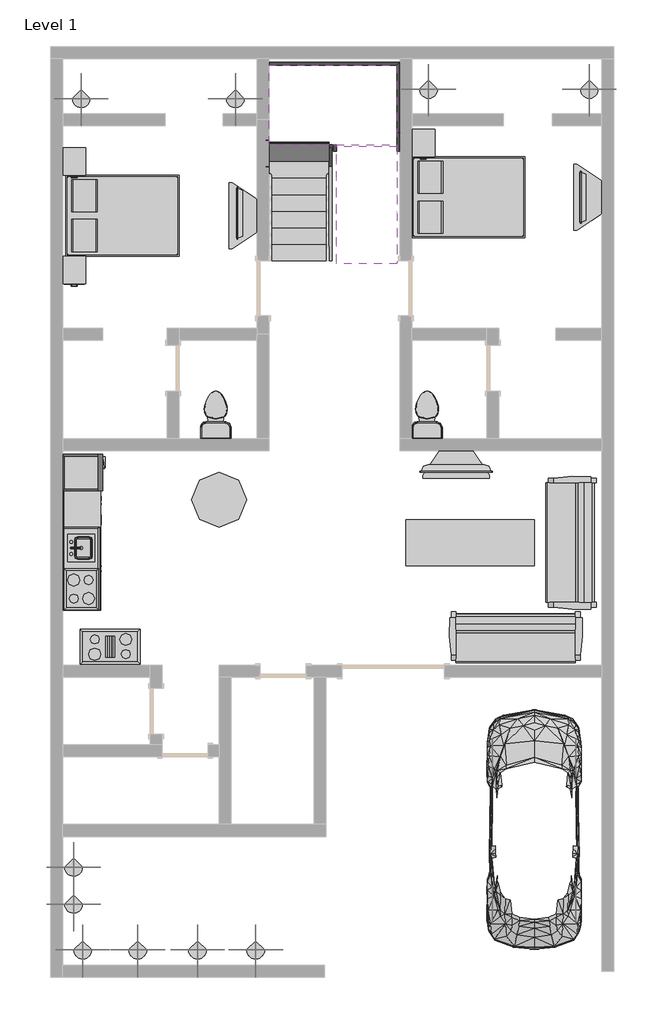
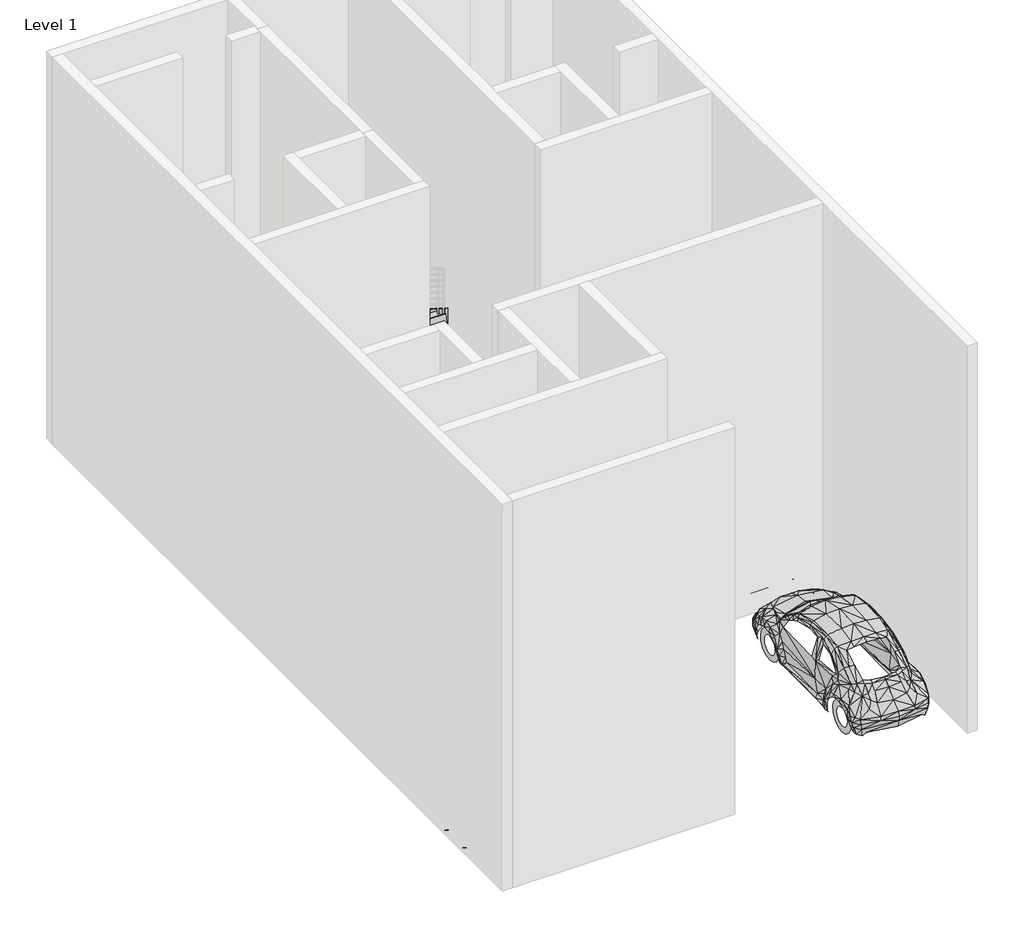
# One storey, part 4 of 4: 16 furniture elements, 10 geographic elements, 8 members, 6 proxies, 3 flow terminals, 2 stair flights, 1 slab.
"""IFC4 building model written with IfcOpenShell, lengths in millimetres."""

from ifc_helpers import new_model, si_unit, frame, origin, place, context, project, spatial, polyline, outline, extrude, faceted_brep, transform, mapped, element, save
from components import m_cook_top_4_unit_0915_x_500mm_0d6b06ed, m_cook_top_4_unit2_0615_x_500mm_249f3515, m_dishwasher_610_x_610_x_875mm_54ecfc4c, m_kitchenette_medium_1372mm_e05c6bec, m_rpc_beetle_m_rpc_beetle_b6d71803, m_refrigerator_600_x_660mm_a466bf94, m_sink_kitchen_island_450_x_450mm_f969cf2d, m_toilet_domestic_3d_m_toilet_domestic_3d_5cb52bd4, m_toilet_domestic_3d_m_toilet_domestic_3d_183bbd19, furniture_40ec15d9, furniture_0810mm_56245f3a, furniture_1190mm_d9bcc661, m_bed_box_1346_x_1880mm_double_b32eb57e, m_cabinet_file_2_drawer_0380_x_0457mm_9eec7cff, m_counter_top_w_sink_hole_600mm_depth_0a237b63, m_sofa_pensi_2134mm_91f3548c, m_table_dining_0762_x_2134mm_3327233b, m_table_dining_round_w_chairs_0915mm_diameter_5defa876, m_rpc_plant_tropical_agave_0_45_meters_eb57889b, non_monolithic_landing_64e54c11, stair_flight_50mm_tread_25mm_nosing_13mm_riser_88d6afc4, stair_flight_50mm_tread_25mm_nosing_13mm_riser_daaaf0ad

model = new_model("IFC4")

# Units and contexts
model_context = context("Model", 3, world=origin())
ifc_project = project(units=[si_unit("LENGTHUNIT", "METRE", prefix="MILLI")], contexts=[model_context])

# Site, building, storey
site = spatial("IfcSite", under=ifc_project)
building = spatial("IfcBuilding", under=site)
storey = spatial("IfcBuildingStorey", under=building, Name="Level 1", Elevation=0.0)

# Proxies
placement = place(None, origin())
m_cook_top_4_unit_0915_x_500mm_shape = m_cook_top_4_unit_0915_x_500mm_0d6b06ed(model_context)
element("IfcBuildingElementProxy", 1, Name="M_Cook Top-4 Unit : 0915 x 500mm", ObjectType="M_Cook Top-4 Unit : 0915 x 500mm", at=placement, inside=storey, context=model_context, shape_type="MappedRepresentation", body=[
    mapped(m_cook_top_4_unit_0915_x_500mm_shape, transform((-7196.5697318, 2497.9482221, 0.0), x_axis=(1.0, 0.0, 0.0), y_axis=(0.0, 1.0, 0.0), z_axis=(0.0, 0.0, 1.0))),
])
m_cook_top_4_unit2_0615_x_500mm_shape = m_cook_top_4_unit2_0615_x_500mm_249f3515(model_context)
element("IfcBuildingElementProxy", 2, Name="M_Cook Top-4 Unit2 : 0615 x 500mm", ObjectType="M_Cook Top-4 Unit2 : 0615 x 500mm", at=placement, inside=storey, context=model_context, shape_type="MappedRepresentation", body=[
    mapped(m_cook_top_4_unit2_0615_x_500mm_shape, transform((-7678.9697318, 3450.1482221, 0.0), x_axis=(0.0, 1.0000000000000002, 0.0), y_axis=(-1.0000000000000002, 0.0, 0.0), z_axis=(0.0, 0.0, 1.0))),
])
m_dishwasher_610_x_610_x_875mm_shape = m_dishwasher_610_x_610_x_875mm_54ecfc4c(model_context)
element("IfcBuildingElementProxy", 3, Name="M_Dishwasher : 610 x 610 x 875mm", ObjectType="M_Dishwasher : 610 x 610 x 875mm", at=placement, inside=storey, context=model_context, shape_type="MappedRepresentation", body=[
    mapped(m_dishwasher_610_x_610_x_875mm_shape, transform((-7412.320167, 4399.6307536, 0.0), x_axis=(0.0, 1.0000000000000002, 0.0), y_axis=(-1.0000000000000002, 0.0, 0.0), z_axis=(0.0, 0.0, 1.0))),
])
m_kitchenette_medium_1372mm_shape = m_kitchenette_medium_1372mm_e05c6bec(model_context)
element("IfcBuildingElementProxy", 4, Name="M_Kitchenette - Medium : 1372mm", ObjectType="M_Kitchenette - Medium : 1372mm", at=placement, inside=storey, context=model_context, shape_type="MappedRepresentation", body=[
    mapped(m_kitchenette_medium_1372mm_shape, transform((-7983.9697318, 3774.4105172, 0.0), x_axis=(0.0, 1.0000000000000002, 0.0), y_axis=(-1.0000000000000002, 0.0, 0.0), z_axis=(0.0, 0.0, 1.0))),
])
m_rpc_beetle_m_rpc_beetle_shape = m_rpc_beetle_m_rpc_beetle_b6d71803(model_context)
element("IfcBuildingElementProxy", 5, Name="M_RPC Beetle : M_RPC Beetle", ObjectType="M_RPC Beetle : M_RPC Beetle", at=placement, inside=storey, context=model_context, shape_type="MappedRepresentation", body=[
    mapped(m_rpc_beetle_m_rpc_beetle_shape, transform((-159.1697318, -1769.2517779, 0.0), x_axis=(1.0, 0.0, 0.0), y_axis=(0.0, 1.0, 0.0), z_axis=(0.0, 0.0, 1.0))),
])
m_refrigerator_600_x_660mm_shape = m_refrigerator_600_x_660mm_a466bf94(model_context)
element("IfcBuildingElementProxy", 6, Name="M_Refrigerator : 600 x 660mm", ObjectType="M_Refrigerator : 600 x 660mm", at=placement, inside=storey, context=model_context, shape_type="MappedRepresentation", body=[
    mapped(m_refrigerator_600_x_660mm_shape, transform((-7687.7546416, 5440.9493647, 0.0), x_axis=(0.0, 1.0000000000000002, 0.0), y_axis=(-1.0000000000000002, 0.0, 0.0), z_axis=(0.0, 0.0, 1.0))),
])

# Flow terminals
m_sink_kitchen_island_450_x_450mm_shape = m_sink_kitchen_island_450_x_450mm_f969cf2d(model_context)
element("IfcFlowTerminal", 7, ObjectType="M_Sink Kitchen-Island : 450 x 450mm", at=placement, inside=storey, context=model_context, shape_type="MappedRepresentation", body=[
    mapped(m_sink_kitchen_island_450_x_450mm_shape, transform((-7676.6243307, 4120.4589815, 0.0), x_axis=(0.0, 1.0000000000000002, 0.0), y_axis=(-1.0000000000000002, 0.0, 0.0), z_axis=(0.0, 0.0, 1.0))),
])
m_toilet_domestic_3d_m_toilet_domestic_3d_shape = m_toilet_domestic_3d_m_toilet_domestic_3d_5cb52bd4(model_context)
m_toilet_domestic_3d_m_toilet_domestic_3d_2_shape = m_toilet_domestic_3d_m_toilet_domestic_3d_183bbd19(model_context)
element("IfcFlowTerminal", 8, ObjectType="M_Toilet-Domestic-3D : M_Toilet-Domestic-3D", at=placement, inside=storey, context=model_context, shape_type="MappedRepresentation", body=[
    mapped(m_toilet_domestic_3d_m_toilet_domestic_3d_shape, transform((-1937.7737045, 6434.9482221, 0.0), x_axis=(-1.0, 0.0, 0.0), y_axis=(0.0, -1.0, 0.0), z_axis=(0.0, 0.0, 1.0))),
    mapped(m_toilet_domestic_3d_m_toilet_domestic_3d_2_shape, transform((-1937.7737045, 6434.9482221, 0.0), x_axis=(-1.0, 0.0, 0.0), y_axis=(0.0, -1.0, 0.0), z_axis=(0.0, 0.0, 1.0))),
])
element("IfcFlowTerminal", 9, ObjectType="M_Toilet-Domestic-3D : M_Toilet-Domestic-3D", at=placement, inside=storey, context=model_context, shape_type="MappedRepresentation", body=[
    mapped(m_toilet_domestic_3d_m_toilet_domestic_3d_shape, transform((-5444.9657592, 6434.9482221, 0.0), x_axis=(-1.0, 0.0, 0.0), y_axis=(0.0, -1.0, 0.0), z_axis=(0.0, 0.0, 1.0))),
    mapped(m_toilet_domestic_3d_m_toilet_domestic_3d_2_shape, transform((-5444.9657592, 6434.9482221, 0.0), x_axis=(-1.0, 0.0, 0.0), y_axis=(0.0, -1.0, 0.0), z_axis=(0.0, 0.0, 1.0))),
])

# Furniture
furniture_shape = furniture_40ec15d9(model_context)
element("IfcFurniture", 10, at=placement, inside=storey, context=model_context, shape_type="MappedRepresentation", body=[
    mapped(furniture_shape, transform((-4761.3197318, 9773.3362242, 0.0), x_axis=(0.0, -1.0000000000000002, 0.0), y_axis=(1.0000000000000002, 0.0, 0.0), z_axis=(0.0, 0.0, 1.0))),
])
element("IfcFurniture", 11, at=placement, inside=storey, context=model_context, shape_type="MappedRepresentation", body=[
    mapped(furniture_shape, transform((960.0302682, 10078.1362242, 0.0), x_axis=(0.0, -1.0, 0.0), y_axis=(1.0, 0.0, 0.0), z_axis=(0.0, 0.0, 1.0))),
])
element("IfcFurniture", 12, at=placement, inside=storey, context=model_context, shape_type="MappedRepresentation", body=[
    mapped(furniture_shape, transform((-1579.7577339, 5750.7482221, 0.0), x_axis=(1.0, 0.0, 0.0), y_axis=(0.0, 1.0, 0.0), z_axis=(0.0, 0.0, 1.0))),
])
furniture_0810mm_shape = furniture_0810mm_56245f3a(model_context)
element("IfcFurniture", 13, ObjectType="0810mm", at=placement, inside=storey, context=model_context, shape_type="MappedRepresentation", body=[
    mapped(furniture_0810mm_shape, transform((671.4916445, 9949.0037079, 0.0), x_axis=(0.0, -1.0000000000000004, 0.0), y_axis=(1.0000000000000004, 0.0, 0.0), z_axis=(0.0, 0.0, 1.0))),
])
element("IfcFurniture", 14, ObjectType="0810mm", at=placement, inside=storey, context=model_context, shape_type="MappedRepresentation", body=[
    mapped(furniture_0810mm_shape, transform((-5028.259817, 9682.2037079, 0.0), x_axis=(0.0, -1.0, 0.0), y_axis=(1.0, 0.0, 0.0), z_axis=(0.0, 0.0, 1.0))),
])
furniture_1190mm_shape = furniture_1190mm_d9bcc661(model_context)
element("IfcFurniture", 15, ObjectType="1190mm", at=placement, inside=storey, context=model_context, shape_type="MappedRepresentation", body=[
    mapped(furniture_1190mm_shape, transform((-1450.6252177, 5462.2095984, 0.0), x_axis=(1.0, 0.0, 0.0), y_axis=(0.0, 1.0, 0.0), z_axis=(0.0, 0.0, 1.0))),
])
m_bed_box_1346_x_1880mm_double_shape = m_bed_box_1346_x_1880mm_double_b32eb57e(model_context)
element("IfcFurniture", 16, ObjectType="M_Bed-Box : 1346 x 1880mm - Double", at=placement, inside=storey, context=model_context, shape_type="MappedRepresentation", body=[
    mapped(m_bed_box_1346_x_1880mm_double_shape, transform((-7229.59924, 9308.9957631, 0.0), x_axis=(0.0, 1.0, 0.0), y_axis=(-1.0, 0.0, 0.0), z_axis=(0.0, 0.0, 1.0))),
])
element("IfcFurniture", 17, ObjectType="M_Bed-Box : 1346 x 1880mm - Double", at=placement, inside=storey, context=model_context, shape_type="MappedRepresentation", body=[
    mapped(m_bed_box_1346_x_1880mm_double_shape, transform((-1485.59924, 9613.7957631, 0.0), x_axis=(0.0, 1.0, 0.0), y_axis=(-1.0, 0.0, 0.0), z_axis=(0.0, 0.0, 1.0))),
])
m_cabinet_file_2_drawer_0380_x_0457mm_shape = m_cabinet_file_2_drawer_0380_x_0457mm_9eec7cff(model_context)
element("IfcFurniture", 18, ObjectType="M_Cabinet-File 2 Drawer : 0380 x 0457mm", at=placement, inside=storey, context=model_context, shape_type="MappedRepresentation", body=[
    mapped(m_cabinet_file_2_drawer_0380_x_0457mm_shape, transform((-7666.0732848, 10691.7825222, 0.0), x_axis=(1.0, 0.0, 0.0), y_axis=(0.0, 1.0, 0.0), z_axis=(0.0, 0.0, 1.0))),
])
element("IfcFurniture", 19, ObjectType="M_Cabinet-File 2 Drawer : 0380 x 0457mm", at=placement, inside=storey, context=model_context, shape_type="MappedRepresentation", body=[
    mapped(m_cabinet_file_2_drawer_0380_x_0457mm_shape, transform((-7666.0732848, 8888.7825222, 0.0), x_axis=(1.0, 0.0, 0.0), y_axis=(0.0, 1.0, 0.0), z_axis=(0.0, 0.0, 1.0))),
])
element("IfcFurniture", 20, ObjectType="M_Cabinet-File 2 Drawer : 0380 x 0457mm", at=placement, inside=storey, context=model_context, shape_type="MappedRepresentation", body=[
    mapped(m_cabinet_file_2_drawer_0380_x_0457mm_shape, transform((-1873.2732848, 10996.5825222, 0.0), x_axis=(1.0, 0.0, 0.0), y_axis=(0.0, 1.0, 0.0), z_axis=(0.0, 0.0, 1.0))),
])
m_counter_top_w_sink_hole_600mm_depth_shape = m_counter_top_w_sink_hole_600mm_depth_0a237b63(model_context)
element("IfcFurniture", 21, ObjectType="M_Counter Top w Sink Hole : 600mm Depth", at=placement, inside=storey, context=model_context, shape_type="MappedRepresentation", body=[
    mapped(m_counter_top_w_sink_hole_600mm_depth_shape, transform((-7983.9697318, 4307.6105172, 0.0), x_axis=(0.0, 1.0000000000000002, 0.0), y_axis=(-1.0000000000000002, 0.0, 0.0), z_axis=(0.0, 0.0, 1.0))),
])
m_sofa_pensi_2134mm_shape = m_sofa_pensi_2134mm_91f3548c(model_context)
element("IfcFurniture", 22, ObjectType="M_Sofa-Pensi : 2134mm", at=placement, inside=storey, context=model_context, shape_type="MappedRepresentation", body=[
    mapped(m_sofa_pensi_2134mm_shape, transform((173.3204321, 4502.1544721, 0.0), x_axis=(0.0, -1.0000000000000004, 0.0), y_axis=(1.0000000000000004, 0.0, 0.0), z_axis=(0.0, 0.0, 1.0))),
])
element("IfcFurniture", 23, ObjectType="M_Sofa-Pensi : 2134mm", at=placement, inside=storey, context=model_context, shape_type="MappedRepresentation", body=[
    mapped(m_sofa_pensi_2134mm_shape, transform((-742.5759818, 2373.238386, 0.0), x_axis=(1.0, 0.0, 0.0), y_axis=(0.0, 1.0, 0.0), z_axis=(0.0, 0.0, 1.0))),
])
m_table_dining_0762_x_2134mm_shape = m_table_dining_0762_x_2134mm_3327233b(model_context)
element("IfcFurniture", 24, ObjectType="M_Table-Dining : 0762 x 2134mm", at=placement, inside=storey, context=model_context, shape_type="MappedRepresentation", body=[
    mapped(m_table_dining_0762_x_2134mm_shape, transform((-1206.1039651, 4318.7592999, 0.0), x_axis=(-1.0, 0.0, 0.0), y_axis=(0.0, -1.0, 0.0), z_axis=(0.0, 0.0, 1.0))),
])
m_table_dining_round_w_chairs_0915mm_diameter_shape = m_table_dining_round_w_chairs_0915mm_diameter_5defa876(model_context)
element("IfcFurniture", 25, ObjectType="M_Table-Dining Round w Chairs : 0915mm Diameter", at=placement, inside=storey, context=model_context, shape_type="MappedRepresentation", body=[
    mapped(m_table_dining_round_w_chairs_0915mm_diameter_shape, transform((-5495.251699, 5121.2269106, 0.0), x_axis=(1.0, 0.0, 0.0), y_axis=(0.0, 1.0, 0.0), z_axis=(0.0, 0.0, 1.0))),
])

# Geographic elements
m_rpc_plant_tropical_agave_0_45_meters_shape = m_rpc_plant_tropical_agave_0_45_meters_eb57889b(model_context)
element("IfcGeographicElement", 26, ObjectType="M_RPC Plant - Tropical : Agave - 0.45 Meters", at=placement, inside=storey, context=model_context, shape_type="MappedRepresentation", body=[
    mapped(m_rpc_plant_tropical_agave_0_45_meters_shape, transform((-7653.9664029, -2531.2517779, 0.0), x_axis=(1.0, 0.0, 0.0), y_axis=(0.0, 1.0, 0.0), z_axis=(0.0, 0.0, 1.0))),
])
element("IfcGeographicElement", 27, ObjectType="M_RPC Plant - Tropical : Agave - 0.45 Meters", at=placement, inside=storey, context=model_context, shape_type="MappedRepresentation", body=[
    mapped(m_rpc_plant_tropical_agave_0_45_meters_shape, transform((-6739.5664029, -2531.2517779, 0.0), x_axis=(1.0, 0.0, 0.0), y_axis=(0.0, 1.0, 0.0), z_axis=(0.0, 0.0, 1.0))),
])
element("IfcGeographicElement", 28, ObjectType="M_RPC Plant - Tropical : Agave - 0.45 Meters", at=placement, inside=storey, context=model_context, shape_type="MappedRepresentation", body=[
    mapped(m_rpc_plant_tropical_agave_0_45_meters_shape, transform((-5748.9664029, -2531.2517779, 0.0), x_axis=(1.0, 0.0, 0.0), y_axis=(0.0, 1.0, 0.0), z_axis=(0.0, 0.0, 1.0))),
])
element("IfcGeographicElement", 29, ObjectType="M_RPC Plant - Tropical : Agave - 0.45 Meters", at=placement, inside=storey, context=model_context, shape_type="MappedRepresentation", body=[
    mapped(m_rpc_plant_tropical_agave_0_45_meters_shape, transform((-4782.1664029, -2531.2517779, 0.0), x_axis=(1.0, 0.0, 0.0), y_axis=(0.0, 1.0, 0.0), z_axis=(0.0, 0.0, 1.0))),
])
element("IfcGeographicElement", 30, ObjectType="M_RPC Plant - Tropical : Agave - 0.45 Meters", at=placement, inside=storey, context=model_context, shape_type="MappedRepresentation", body=[
    mapped(m_rpc_plant_tropical_agave_0_45_meters_shape, transform((-7806.3664029, -1159.6517779, 0.0), x_axis=(1.0, 0.0, 0.0), y_axis=(0.0, 1.0, 0.0), z_axis=(0.0, 0.0, 1.0))),
])
element("IfcGeographicElement", 31, ObjectType="M_RPC Plant - Tropical : Agave - 0.45 Meters", at=placement, inside=storey, context=model_context, shape_type="MappedRepresentation", body=[
    mapped(m_rpc_plant_tropical_agave_0_45_meters_shape, transform((-7806.3664029, -1769.2517779, 0.0), x_axis=(1.0, 0.0, 0.0), y_axis=(0.0, 1.0, 0.0), z_axis=(0.0, 0.0, 1.0))),
])
element("IfcGeographicElement", 32, ObjectType="M_RPC Plant - Tropical : Agave - 0.45 Meters", at=placement, inside=storey, context=model_context, shape_type="MappedRepresentation", body=[
    mapped(m_rpc_plant_tropical_agave_0_45_meters_shape, transform((-7679.3664029, 11591.1482221, 0.0), x_axis=(1.0, 0.0, 0.0), y_axis=(0.0, 1.0, 0.0), z_axis=(0.0, 0.0, 1.0))),
])
element("IfcGeographicElement", 33, ObjectType="M_RPC Plant - Tropical : Agave - 0.45 Meters", at=placement, inside=storey, context=model_context, shape_type="MappedRepresentation", body=[
    mapped(m_rpc_plant_tropical_agave_0_45_meters_shape, transform((-5120.3164029, 11591.1482221, 0.0), x_axis=(1.0, 0.0, 0.0), y_axis=(0.0, 1.0, 0.0), z_axis=(0.0, 0.0, 1.0))),
])
element("IfcGeographicElement", 34, ObjectType="M_RPC Plant - Tropical : Agave - 0.45 Meters", at=placement, inside=storey, context=model_context, shape_type="MappedRepresentation", body=[
    mapped(m_rpc_plant_tropical_agave_0_45_meters_shape, transform((-1911.9664029, 11743.5482221, 0.0), x_axis=(1.0, 0.0, 0.0), y_axis=(0.0, 1.0, 0.0), z_axis=(0.0, 0.0, 1.0))),
])
element("IfcGeographicElement", 35, ObjectType="M_RPC Plant - Tropical : Agave - 0.45 Meters", at=placement, inside=storey, context=model_context, shape_type="MappedRepresentation", body=[
    mapped(m_rpc_plant_tropical_agave_0_45_meters_shape, transform((755.0335971, 11743.5482221, 0.0), x_axis=(1.0, 0.0, 0.0), y_axis=(0.0, 1.0, 0.0), z_axis=(0.0, 0.0, 1.0))),
])

# Members
element("IfcMember", 36, ObjectType="Stringer - 50mm Width", at=placement, inside=storey, context=model_context, shape_type="SweptSolid", body=[
    extrude(outline(polyline([(8898.7482221, 0.0), (8898.7482221, 215.089535), (10833.5792256, 1438.6980748), (10949.4482857, 1038.6980748), (9307.0069549, 0.0), (8898.7482221, 0.0)])), frame((-4612.9197318, 0.0, 0.0), z_axis=(1.0, 0.0, 0.0), x_axis=(0.0, 1.0, 0.0)), (0.0, 0.0, 1.0), 50.0),
])
element("IfcMember", 37, ObjectType="Stringer - 50mm Width", at=placement, inside=storey, context=model_context, shape_type="SweptSolid", body=[
    extrude(outline(polyline([(8898.7482221, 0.0), (8898.7482221, 215.089535), (10773.7482221, 1400.860286), (10773.7482221, 927.5834101), (9307.0069549, 0.0), (8898.7482221, 0.0)])), frame((-3562.8939506, 0.0, 0.0), z_axis=(1.0, 0.0, 0.0), x_axis=(0.0, 1.0, 0.0)), (0.0, 0.0, 1.0), 50.0),
])
element("IfcMember", 38, ObjectType="Stringer - 50mm Width", at=placement, inside=storey, context=model_context, shape_type="SweptSolid", body=[
    extrude(outline(polyline([(11088.9172185, 1438.6980748), (10973.0481585, 1038.6980748), (8898.7482221, 2350.5083113), (8898.7482221, 2823.7851872), (11088.9172185, 1438.6980748)])), frame((-2440.2681693, 0.0, 0.0), z_axis=(1.0, 0.0, 0.0), x_axis=(0.0, 1.0, 0.0)), (0.0, 0.0, 1.0), 50.0),
])
element("IfcMember", 39, ObjectType="Stringer - 50mm Width", at=placement, inside=storey, context=model_context, shape_type="SweptSolid", body=[
    extrude(outline(polyline([(10823.7482221, 1606.3938828), (10823.7482221, 1133.1170069), (8898.7482221, 2350.5083113), (8898.7482221, 2823.7851872), (10823.7482221, 1606.3938828)])), frame((-3490.2939506, 0.0, 0.0), z_axis=(1.0, 0.0, 0.0), x_axis=(0.0, 1.0, 0.0)), (0.0, 0.0, 1.0), 50.0),
])
element("IfcMember", 40, ObjectType="Stringer - 50mm Width", at=placement, inside=storey, context=model_context, shape_type="Brep", body=[
    faceted_brep([(-2440.2681693, 11088.9172185, 1438.6980748), (-2390.2681693, 11088.9172185, 1438.6980748), (-2390.2681693, 12194.5482221, 1438.6980748), (-2440.2681693, 12144.5482221, 1438.6980748), (-2440.2681693, 10973.0481585, 1038.6980748), (-2440.2681693, 12144.5482221, 1038.6980748), (-2390.2681693, 10973.0481585, 1038.6980748), (-2390.2681693, 12194.5482221, 1038.6980748)], [[[0, 1, 2, 3]], [[4, 0, 3, 5]], [[6, 4, 5, 7]], [[1, 6, 7, 2]], [[1, 0, 4, 6]], [[2, 7, 5, 3]]]),
])
element("IfcMember", 41, ObjectType="Stringer - 50mm Width", at=placement, inside=storey, context=model_context, shape_type="SweptSolid", body=[
    extrude(outline(polyline([(-2390.2681693, 12194.5482221), (-2440.2681693, 12144.5482221), (-4562.9197318, 12144.5482221), (-4612.9197318, 12194.5482221), (-2390.2681693, 12194.5482221)])), frame((0.0, 0.0, 1038.6980748), z_axis=(0.0, 0.0, 1.0), x_axis=(1.0, 0.0, 0.0)), (0.0, 0.0, 1.0), 400.0),
])
element("IfcMember", 42, ObjectType="Stringer - 50mm Width", at=placement, inside=storey, context=model_context, shape_type="Brep", body=[
    faceted_brep([(-4562.9197318, 12144.5482221, 1438.6980748), (-4612.9197318, 12194.5482221, 1438.6980748), (-4612.9197318, 10833.5792256, 1438.6980748), (-4562.9197318, 10833.5792256, 1438.6980748), (-4562.9197318, 12144.5482221, 1038.6980748), (-4562.9197318, 10949.4482857, 1038.6980748), (-4612.9197318, 12194.5482221, 1038.6980748), (-4612.9197318, 10949.4482857, 1038.6980748)], [[[0, 1, 2, 3]], [[4, 0, 3, 5]], [[6, 4, 5, 7]], [[1, 6, 7, 2]], [[1, 0, 4, 6]], [[2, 7, 5, 3]]]),
])
element("IfcMember", 43, ObjectType="Stringer - 50mm Width", at=placement, inside=storey, context=model_context, shape_type="SweptSolid", body=[
    extrude(outline(polyline([(-3562.8939506, 10773.7482221), (-3562.8939506, 10823.7482221), (-3490.2939506, 10823.7482221), (-3490.2939506, 10773.7482221), (-3562.8939506, 10773.7482221)])), frame((0.0, 0.0, 1038.6980748), z_axis=(0.0, 0.0, 1.0), x_axis=(1.0, 0.0, 0.0)), (0.0, 0.0, 1.0), 400.0),
])

# Slab
non_monolithic_landing_shape = non_monolithic_landing_64e54c11(model_context)
element("IfcSlab", 44, ObjectType="Non-Monolithic Landing", at=placement, inside=storey, context=model_context, shape_type="MappedRepresentation", body=[
    mapped(non_monolithic_landing_shape, transform((0.0, 0.0, 0.0), x_axis=(1.0, 0.0, 0.0), y_axis=(0.0, 1.0, 0.0), z_axis=(0.0, 0.0, 1.0))),
])

# Stair flights
stair_flight_50mm_tread_25mm_nosing_13mm_riser_shape = stair_flight_50mm_tread_25mm_nosing_13mm_riser_88d6afc4(model_context)
element("IfcStairFlight", 45, ObjectType="50mm Tread 25mm Nosing 13mm Riser", at=placement, inside=storey, context=model_context, shape_type="MappedRepresentation", body=[
    mapped(stair_flight_50mm_tread_25mm_nosing_13mm_riser_shape, transform((0.0, 0.0, 0.0), x_axis=(1.0, 0.0, 0.0), y_axis=(0.0, 1.0, 0.0), z_axis=(0.0, 0.0, 1.0))),
])
stair_flight_50mm_tread_25mm_nosing_13mm_riser_2_shape = stair_flight_50mm_tread_25mm_nosing_13mm_riser_daaaf0ad(model_context)
element("IfcStairFlight", 46, ObjectType="50mm Tread 25mm Nosing 13mm Riser", at=placement, inside=storey, context=model_context, shape_type="MappedRepresentation", body=[
    mapped(stair_flight_50mm_tread_25mm_nosing_13mm_riser_2_shape, transform((0.0, 0.0, 0.0), x_axis=(1.0, 0.0, 0.0), y_axis=(0.0, 1.0, 0.0), z_axis=(0.0, 0.0, 1.0))),
])

save(model, "model.ifc")

# Revit data of these elements
# Type "M_Cook Top-4 Unit : 0915 x 500mm"
#   Counter Height = 900 mm
#   Depth = 500 mm
#   Width = 915 mm
#   Burner Material = Steel, Chrome Plated
#   Cooktop Material = Steel, Polished
#   Default Elevation = 0
# Type "M_Cook Top-4 Unit2 : 0615 x 500mm"
#   Depth = 500 mm
#   Width = 615 mm
#   Burner Material = Steel, Chrome Plated
#   Cooktop Material = Steel, Polished
#   Default Elevation = 0
#   Assembly Code = ""
# Type "M_Dishwasher : 610 x 610 x 875mm"
#   Label = "DW"
#   Depth = 610 mm
#   Height = 875 mm
#   Width = 610 mm
#   Dishwasher Material = Steel, Paint Finish, Ivory, Glossy
#   Panel Face Material = Plastic, Opaque Black
#   Default Elevation = 0
# Type "M_Kitchenette - Medium : 1372mm"
#   Counter Length = 1980 mm
#   Cabinet Width = 1372 mm
#   Cabinet Height = 900 mm
#   Cabinet Depth = 610 mm
#   Toe Depth = 35 mm
#   Toe Height = 100 mm
#   Cabinet Material = Cabinets
#   Door/Drawer Material = Cabinets
#   Handle Material = Cabinets - Handles
#   Default Elevation = 0
# Type "M_RPC Beetle : M_RPC Beetle"
#   built-in parameter 1005198 = "{2, 15},{39, RPC-16-0U6E-L4EG-ENH1-J3KF-SVEL-0TX4-C0},{1, 0},{1, 0},{2, 18},{1, 8},{5, Color},{1, 0},{1, 0},{3, 0.8},{3, 0.8},{3, 0.8},{1, 8},{7, BBoxMin},{1, 0},{1, 0},{1, 0},{1, 0},{1, 0},{1, 8},{7, BBoxMax},{1, 0},{1, 0},{1, 0},{1, 0},{1, 0},{2, 11},{9, RPCTypeId},{1, 0},{1, 0},{39, RPC-16-0U6E-L4EG-ENH1-J3KF-SVEL-0TX4-C0},{1, 6},{14, RPCPlantHeight},{1, 0},{1, 0},{4, 4.92},{2, 11},{7, keyword},{1, 0},{1, 0},{39, :RPCs:Auto_Economy/Midsize:Geometry:RPC},{2, 11},{8, category},{1, 0},{1, 0},{20, Auto_Economy/Midsize},{2, 11},{12, LocalizedUID},{1, 0},{1, 0},{13, VW Beetle [4]},{2, 14},{6, Height},{1, 0},{1, 0},{4, 4.92},{1, 2},{16, Cast Reflections},{1, 0},{1, 0},{1, 0},{1, 4},{12, Transparency},{1, 0},{1, 0},{2, 18},{1, 4},{7, Tinting},{1, 0},{1, 0},{2, 50},{1, 2},{11, Use Tinting},{1, 0},{1, 0},{1, 0},{1, 2},{13, License Plate},{1, 0},{1, 0},{1, 0},{2, 11},{21, License Plate Texture},{1, 0},{1, 0},{64, __RPC:/object data/textures/car/plate/textures/default/rgb/0/0/0},{2, 11},{23, i_License Plate Texture},{1, 0},{1, 0},{0, },{1, 2},{12, Custom Plate},{1, 0},{1, 0},{1, 0},{2, 11},{23, License Plate File Name},{1, 0},{1, 0},{0, },{21, assetlibrary_base.fbx},{1, 5},"
#   built-in parameter 1005195 = "RPC-16-0U6E-L4EG-ENH1-J3KF-SVEL-0TX4-C0"
#   Height = 0
# Type "M_Refrigerator : 600 x 660mm"
#   Label = "REF."
#   Depth = 660 mm
#   Height = 1830 mm
#   Width = 600 mm
#   Material = Steel, Paint Finish, Ivory, Matte
#   Description = (empty or 0)
#   Default Elevation = 0
# Type "M_Sink Kitchen-Island : 450 x 450mm"
#   Counter Height [instance default] = 900 mm
#   Depth = 450 mm
#   Width = 450 mm
#   Fixture Material = Steel, Polished
#   Sink Material = Steel, Polished
#   Default Elevation = 0
# Type "M_Toilet-Domestic-3D : M_Toilet-Domestic-3D"
#   Bowl/Basin Material = Porcelain, Linen
#   Seat Material = Laminate, Linen, Matte
#   Default Elevation = 0
# Type
#   Depth = 460 mm
#   Width = 1100 mm
#   Height = 500 mm
#   Finish = Melamine - Gray
#   Default Elevation = 0
# Type "0810mm"
#   SinAng = 0.49 mm
#   L = 705.961 mm
#   H = 397.139 mm
#   Thickness = 110 mm
#   Diagonal = 810 mm
#   CosAng = 0.872 mm
#   Stand [instance default] = yes
#   Default Elevation = 0
# Type "1190mm"
#   SinAng = 0.49 mm
#   L = 1037.152 mm
#   H = 583.452 mm
#   Thickness = 110 mm
#   Diagonal = 1190 mm
#   CosAng = 0.872 mm
#   Stand [instance default] = yes
#   Default Elevation = 0
# Type "M_Bed-Box : 1346 x 1880mm - Double"
#   Length = 1880 mm
#   Width = 1346 mm
#   Frame Material = Birch
#   Mattress Material = Linen, White
#   Default Elevation = 0
# Type "M_Cabinet-File 2 Drawer : 0380 x 0457mm"
#   Depth = 457 mm
#   Height = 734 mm
#   Width = 380 mm
#   Cabinet Material = Steel, Paint Finish, Ivory, Glossy
#   Handle Material = Steel, Chrome Plated
#   Default Elevation = 0
# Type "M_Counter Top w Sink Hole : 600mm Depth"
#   Counter Thickness = 40 mm
#   Depth = 625 mm
#   Height = 900 mm
#   Length [instance default] = 2500 mm
#   Sink Location [instance default] = 1200 mm
#   Sink Location To Wall [instance default] = 100 mm
#   Sink Opening Depth [instance default] = 378 mm
#   Sink Opening Width [instance default] = 587 mm
#   Counter Top Material = none
#   Default Elevation = 0
# Type "M_Sofa-Pensi : 2134mm"
#   Length = 2134 mm
#   Sofa Material = Linen, Beige
#   Frame Material = Steel, Chrome Plated
#   Default Elevation = 0
# Type "M_Table-Dining : 0762 x 2134mm"
#   Height = 560 mm
#   Length = 2134 mm
#   Width = 762 mm
#   Base Material = Steel, Chrome Plated
#   Top Material = Glass - Clear, Grey
#   Default Elevation = 0
# Type "M_Table-Dining Round w Chairs : 0915mm Diameter"
#   Radius = 457.5 mm
#   Diameter = 915 mm
#   Height = 762 mm
#   Chairs = 4
#   Base Material = Pine
#   Top Material = Laminate, Linen, Matte
#   Default Elevation = 0
# Type "M_RPC Plant - Tropical : Agave - 0.45 Meters"
#   built-in parameter 1005198 = "{2, 15},{39, RPC-16-G1GJ-63FX-7K5P-N000-ST1L-LVER-AU},{1, 0},{1, 0},{2, 13},{1, 8},{5, Color},{1, 0},{1, 0},{3, 0.8},{3, 0.8},{3, 0.8},{1, 8},{7, BBoxMin},{1, 0},{1, 0},{1, 0},{1, 0},{1, 0},{1, 8},{7, BBoxMax},{1, 0},{1, 0},{1, 0},{1, 0},{1, 0},{2, 11},{9, RPCTypeId},{1, 0},{1, 0},{39, RPC-16-G1GJ-63FX-7K5P-N000-ST1L-LVER-AU},{1, 6},{14, RPCPlantHeight},{1, 0},{1, 0},{7, 1.47638},{2, 11},{7, keyword},{1, 0},{1, 0},{35, :RPCs:Plants [General]:Geometry:RPC},{2, 11},{8, category},{1, 0},{1, 0},{16, Plants [General]},{2, 11},{12, LocalizedUID},{1, 0},{1, 0},{5, Agave},{2, 14},{6, Height},{1, 0},{1, 0},{7, 1.47638},{1, 2},{16, Cast Reflections},{1, 0},{1, 0},{1, 0},{1, 2},{12, Cast Shadows},{1, 0},{1, 0},{1, 1},{1, 2},{9, Lock View},{1, 0},{1, 0},{1, 0},{1, 4},{5, ViewC},{1, 0},{1, 0},{1, 0},{21, assetlibrary_base.fbx},{1, 5},"
#   built-in parameter 1005195 = "RPC-16-G1GJ-63FX-7K5P-N000-ST1L-LVER-AU"
#   Type Comments = "Agave"
#   Height = 450 mm
#   Description = (empty or 0)
#   Default Elevation = 0
# Element 1 (IfcBuildingElementProxy, "M_Cook Top-4 Unit : 0915 x 500mm")
#   Phase Created = New Construction
#   Materials on its faces: "Steel, Chrome Plated", "Steel, Polished"
# Element 2 (IfcBuildingElementProxy, "M_Cook Top-4 Unit2 : 0615 x 500mm")
#   Phase Created = New Construction
#   Materials on its faces: "Steel, Polished", "Steel, Chrome Plated"
# Element 3 (IfcBuildingElementProxy, "M_Dishwasher : 610 x 610 x 875mm")
#   Phase Created = New Construction
#   Materials on its faces: "Steel, Paint Finish, Ivory, Glossy", "Plastic, Opaque Black"
# Element 4 (IfcBuildingElementProxy, "M_Kitchenette - Medium : 1372mm")
#   Phase Created = New Construction
#   Materials on its faces: "Cabinets", "Cabinets - Handles"
# Element 5 (IfcBuildingElementProxy, "M_RPC Beetle : M_RPC Beetle")
#   Phase Created = New Construction
# Element 6 (IfcBuildingElementProxy, "M_Refrigerator : 600 x 660mm")
#   Phase Created = New Construction
#   Materials on its faces: "Steel, Paint Finish, Ivory, Matte", "Steel, Chrome Plated"
# Element 7 (IfcFlowTerminal, "M_Sink Kitchen-Island : 450 x 450mm")
#   Mark = "3"
#   Counter Height = 900 mm
#   Phase Created = New Construction
#   Materials on its faces: "Steel, Polished"
# Element 8 (IfcFlowTerminal, "M_Toilet-Domestic-3D : M_Toilet-Domestic-3D")
#   Mark = "1"
#   Phase Created = New Construction
#   Materials on its faces: "Porcelain, Linen", "Laminate, Linen, Matte"
# Element 9 (IfcFlowTerminal, "M_Toilet-Domestic-3D : M_Toilet-Domestic-3D")
#   Mark = "2"
#   Phase Created = New Construction
#   Materials on its faces: "Porcelain, Linen", "Laminate, Linen, Matte"
# Elements 10, 11, 12 (IfcFurniture)
#   Phase Created = New Construction
#   Materials on its faces: "Melamine - Gray", "Glass - Shelves"
# Elements 13, 14 (IfcFurniture, "0810mm")
#   Stand = yes
#   Phase Created = New Construction
#   Materials on its faces: "TV - Black", "TV - Glass", "TV - Screen"
# Element 15 (IfcFurniture, "1190mm")
#   Stand = yes
#   Phase Created = New Construction
#   Materials on its faces: "TV - Black", "TV - Glass", "TV - Screen"
# Elements 16, 17 (IfcFurniture, "M_Bed-Box : 1346 x 1880mm - Double")
#   Phase Created = New Construction
#   Materials on its faces: "Birch", "Linen, White"
# Elements 18, 19, 20 (IfcFurniture, "M_Cabinet-File 2 Drawer : 0380 x 0457mm")
#   Phase Created = New Construction
#   Materials on its faces: "Steel, Chrome Plated", "Steel, Paint Finish, Ivory, Glossy"
# Element 21 (IfcFurniture, "M_Counter Top w Sink Hole : 600mm Depth")
#   Sink Opening Width = 400 mm
#   Sink Opening Depth = 350 mm
#   Sink Location To Wall = 160 mm
#   Sink Location = 1025 mm
#   Length = 1980 mm
#   Phase Created = New Construction
#   Materials on its faces: "Counter Top"
# Elements 22, 23 (IfcFurniture, "M_Sofa-Pensi : 2134mm")
#   Phase Created = New Construction
#   Materials on its faces: "Linen, Beige", "Steel, Chrome Plated"
# Element 24 (IfcFurniture, "M_Table-Dining : 0762 x 2134mm")
#   Phase Created = New Construction
#   Materials on its faces: "Steel, Chrome Plated", "Glass - Clear, Grey"
# Element 25 (IfcFurniture, "M_Table-Dining Round w Chairs : 0915mm Diameter")
#   Phase Created = New Construction
#   Materials on its faces: "Pine", "Laminate, Linen, Matte"
# Elements 26, 27, 28, 29, 30, 31, 32, 33, 34, 35 (IfcGeographicElement, "M_RPC Plant - Tropical : Agave - 0.45 Meters")
#   Phase Created = New Construction
# Elements 36, 37, 38, 39, 40, 41, 42, 43 (IfcMember, "Stringer - 50mm Width")
#   Phase Created = New Construction
# Element 44 (IfcSlab, "Non-Monolithic Landing")
#   Phase Created = New Construction
# Elements 45, 46 (IfcStairFlight, "50mm Tread 25mm Nosing 13mm Riser")
#   Phase Created = New Construction
# Materials
#   "Steel, Chrome Plated": class "Metal", colour RGB 244 244 244, transparency 0, Description = "Chromiuim plated steel", Cost = 0
#   "Steel, Polished": class "Metal", colour RGB 57 57 57, transparency 0, Description = "Polished steel", Cost = 0
#   "Steel, Paint Finish, Ivory, Glossy": class "Metal", colour RGB 247 247 239, transparency 0, Description = "Steel, paint finish, ivory, glossy", Cost = 0
#   "Plastic, Opaque Black": class "Plastic", colour RGB 0 0 0, transparency 0.7, Description = "Plastic, generic, opaque black", Cost = 0
#   "Cabinets": colour RGB 249 249 249, transparency 0
#   "Cabinets - Handles": class "Metal", colour RGB 57 57 57, transparency 0
#   "Steel, Paint Finish, Ivory, Matte": class "Metal", colour RGB 247 247 239, transparency 0, Description = "Steel, paint finish, ivory, matte", Cost = 0
#   "Porcelain, Linen": class "Ceramic", colour RGB 249 239 230, transparency 0, Description = "Porcelain, linen", Cost = 0
#   "Laminate, Linen, Matte": class "Plastic", colour RGB 249 239 230, transparency 0, Description = "Plastic Laminate - Linen, Matte", Cost = 0
#   "Melamine - Gray": class "Wood", colour RGB 49 49 49, transparency 0
#   "Birch": class "Wood", colour RGB 224 178 126, transparency 0, Description = "Betula Alleghaniensis", Cost = 0
#   "Linen, White": class "Textile", colour RGB 247 247 239, transparency 0, Description = "Linen, white", Cost = 0
#   "Linen, Beige": class "Textile", colour RGB 249 239 230, transparency 0, Description = "Linen, beige", Cost = 0
#   "Glass - Clear, Grey": class "Glass", colour RGB 252 255 255, transparency 0.64
#   "Pine": class "Wood", colour RGB 223 192 134, transparency 0, Description = "Pinus Echinata", Cost = 0
#   "Glass - Shelves": class "Glass", colour RGB 167 167 167, transparency 0.9
#   "TV - Black": colour RGB 49 49 49, transparency 0
#   "TV - Glass": colour RGB 157 157 157, transparency 0.9
#   "TV - Screen": colour RGB 0 0 0, transparency 0
#   "Counter Top": class "Wood", colour RGB 226 177 128, transparency 0
